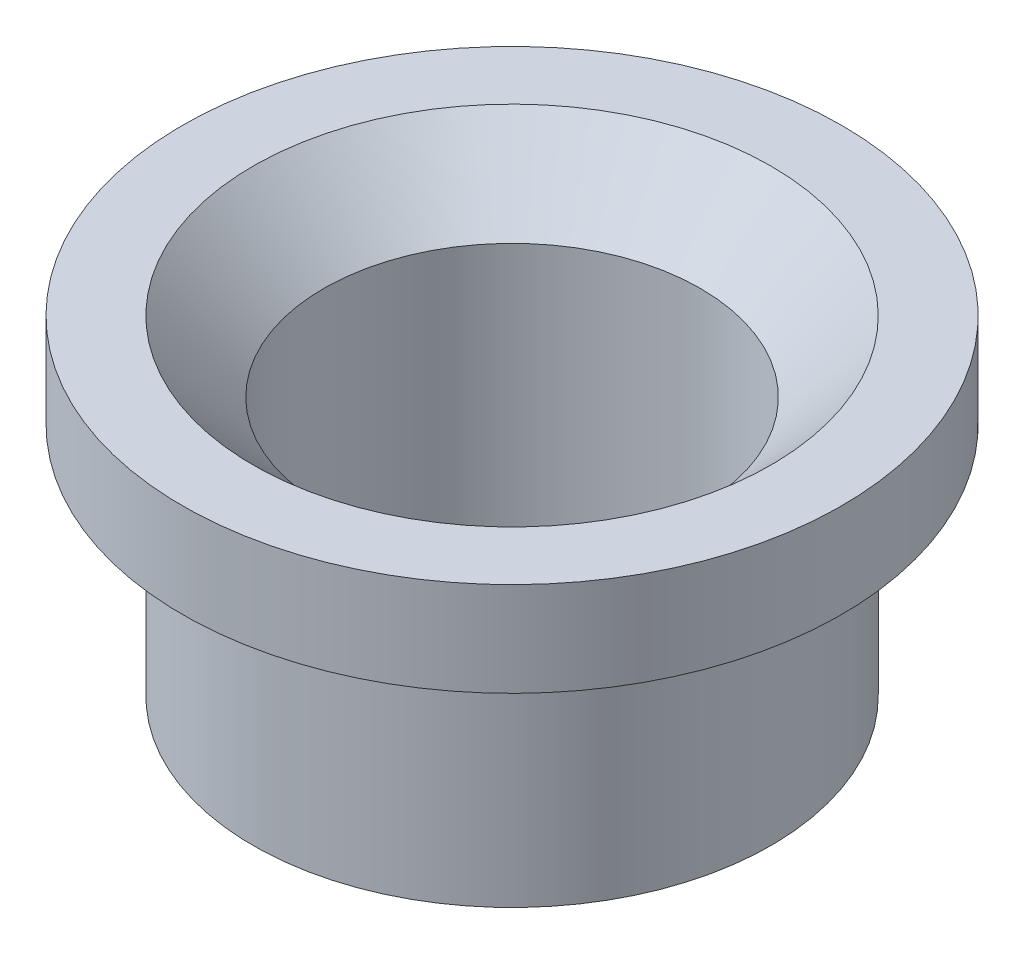
SolidWorks part; units mm, degrees
material "Plain Carbon Steel"
ref_plane "Front Plane" through (0, 0, 0) normal (0, 0, 1) x (1, 0, 0)
ref_plane "Top Plane" through (0, 0, 0) normal (0, 1, 0) x (1, 0, 0)
ref_plane "Right Plane" through (0, 0, 0) normal (1, 0, 0) x (0, 0, -1)
sketch "Bush Half-Section Profile" plane through (0, 0, 0) normal (0, 0, 1) x (1, 0, 0)
  line L0 (12, 0) -> (12, 16.5)
  line L1 (12, 16.5) -> (16.5, 21)
  line L2 (16.5, 21) -> (21, 21)
  line L3 (21, 21) -> (21, 15)
  line L4 (21, 15) -> (16.5, 15)
  line L5 (16.5, 15) -> (16.5, 0)
  line L6 (16.5, 0) -> (12, 0)
  line L7 (0, 0) -> (0, 24.2896) construction
  dimension "D1" = 12
  dimension "D2" = 16.5
  dimension "D3" = 15
  dimension "D4" = 6
  dimension "D5" = 21
  dimension "D6" = 45
  dimension "D7" = 16.5
revolve "Flanged Bush Body" add sketch "Bush Half-Section Profile" angle 360 about L7
